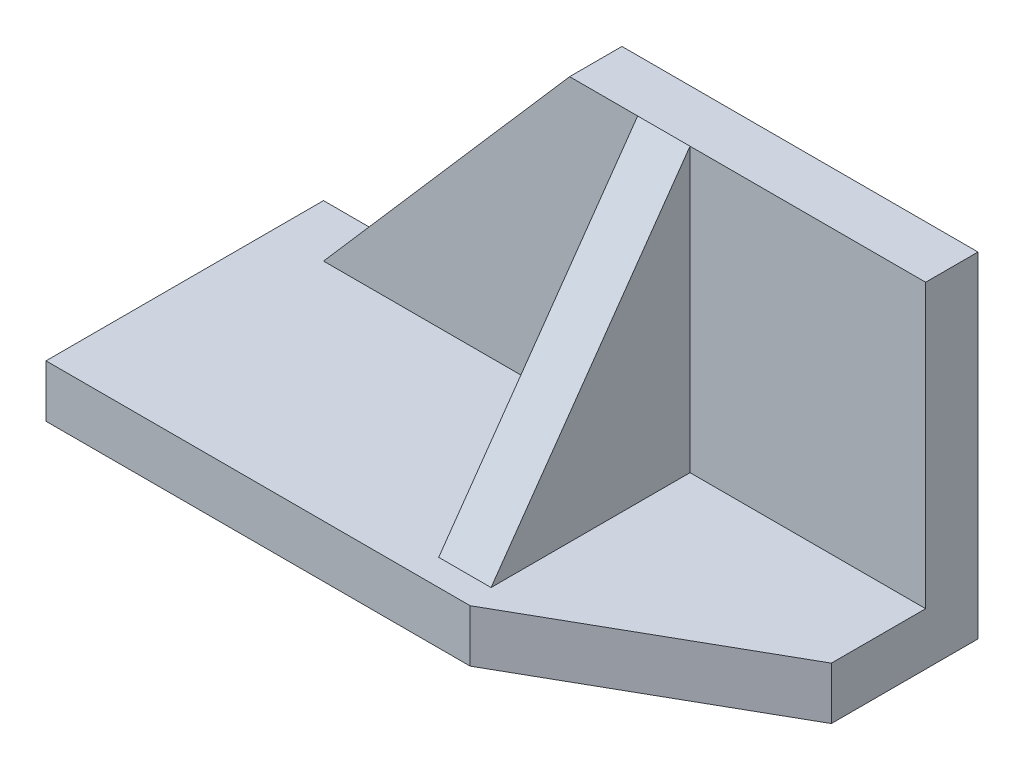
ISO-10303-21;
HEADER;
FILE_DESCRIPTION(('STEP AP214'),'2;1');
FILE_NAME('part.step','',(''),(''),'','','');
FILE_SCHEMA(('AUTOMOTIVE_DESIGN { 1 0 10303 214 1 1 1 1 }'));
ENDSEC;
DATA;
#1=APPLICATION_CONTEXT('core data for automotive mechanical design processes');
#2=APPLICATION_PROTOCOL_DEFINITION('international standard','automotive_design',2000,#1);
#3=PRODUCT_CONTEXT('',#1,'mechanical');
#4=PRODUCT('Part','Part','',(#3));
#5=PRODUCT_RELATED_PRODUCT_CATEGORY('part','',(#4));
#6=PRODUCT_DEFINITION_FORMATION('','',#4);
#7=PRODUCT_DEFINITION_CONTEXT('part definition',#1,'design');
#8=PRODUCT_DEFINITION('design','',#6,#7);
#9=PRODUCT_DEFINITION_SHAPE('','',#8);
#10=(LENGTH_UNIT() NAMED_UNIT(*) SI_UNIT(.MILLI.,.METRE.));
#11=(NAMED_UNIT(*) PLANE_ANGLE_UNIT() SI_UNIT($,.RADIAN.));
#12=(NAMED_UNIT(*) SI_UNIT($,.STERADIAN.) SOLID_ANGLE_UNIT());
#13=UNCERTAINTY_MEASURE_WITH_UNIT(LENGTH_MEASURE(1.E-05),#10,'distance_accuracy_value','');
#14=(GEOMETRIC_REPRESENTATION_CONTEXT(3) GLOBAL_UNCERTAINTY_ASSIGNED_CONTEXT((#13)) GLOBAL_UNIT_ASSIGNED_CONTEXT((#10,
#11,#12)) REPRESENTATION_CONTEXT('',''));
#15=CARTESIAN_POINT('',(0.,0.,0.));
#16=DIRECTION('',(0.,0.,1.));
#17=DIRECTION('',(1.,0.,0.));
#18=AXIS2_PLACEMENT_3D('',#15,#16,#17);
#19=CARTESIAN_POINT('',(0.,5.,0.));
#20=DIRECTION('',(0.,1.,0.));
#21=DIRECTION('',(0.,0.,1.));
#22=AXIS2_PLACEMENT_3D('',#19,#20,#21);
#23=PLANE('',#22);
#24=DIRECTION('',(1.,0.,0.));
#25=VECTOR('',#24,1.);
#26=CARTESIAN_POINT('',(80.,5.,-5.));
#27=LINE('',#26,#25);
#28=CARTESIAN_POINT('',(70.,5.,-5.));
#29=VERTEX_POINT('',#28);
#30=CARTESIAN_POINT('',(80.,5.,-5.));
#31=VERTEX_POINT('',#30);
#32=EDGE_CURVE('E53',#29,#31,#27,.T.);
#33=ORIENTED_EDGE('',*,*,#32,.F.);
#34=DIRECTION('',(0.,0.,1.));
#35=VECTOR('',#34,1.);
#36=CARTESIAN_POINT('',(70.,5.,-5.));
#37=LINE('',#36,#35);
#38=CARTESIAN_POINT('',(70.,5.,-43.));
#39=VERTEX_POINT('',#38);
#40=EDGE_CURVE('E61',#39,#29,#37,.T.);
#41=ORIENTED_EDGE('',*,*,#40,.F.);
#42=DIRECTION('',(-1.,0.,0.));
#43=VECTOR('',#42,1.);
#44=CARTESIAN_POINT('',(125.,5.,-43.));
#45=LINE('',#44,#43);
#46=CARTESIAN_POINT('',(10.,5.,-43.));
#47=VERTEX_POINT('',#46);
#48=EDGE_CURVE('E153',#39,#47,#45,.T.);
#49=ORIENTED_EDGE('',*,*,#48,.T.);
#50=DIRECTION('',(0.,0.,-1.));
#51=VECTOR('',#50,1.);
#52=CARTESIAN_POINT('',(10.,5.,-43.));
#53=LINE('',#52,#51);
#54=CARTESIAN_POINT('',(10.,5.,-53.));
#55=VERTEX_POINT('',#54);
#56=EDGE_CURVE('E164',#47,#55,#53,.T.);
#57=ORIENTED_EDGE('',*,*,#56,.T.);
#58=DIRECTION('',(-1.,0.,0.));
#59=VECTOR('',#58,1.);
#60=CARTESIAN_POINT('',(125.,5.,-53.));
#61=LINE('',#60,#59);
#62=CARTESIAN_POINT('',(0.,5.,-53.));
#63=VERTEX_POINT('',#62);
#64=EDGE_CURVE('E181',#55,#63,#61,.T.);
#65=ORIENTED_EDGE('',*,*,#64,.T.);
#66=DIRECTION('',(0.,0.,1.));
#67=VECTOR('',#66,1.);
#68=CARTESIAN_POINT('',(0.,5.,-53.));
#69=LINE('',#68,#67);
#70=CARTESIAN_POINT('',(0.,5.,0.));
#71=VERTEX_POINT('',#70);
#72=EDGE_CURVE('E172',#63,#71,#69,.T.);
#73=ORIENTED_EDGE('',*,*,#72,.T.);
#74=DIRECTION('',(1.,0.,0.));
#75=VECTOR('',#74,1.);
#76=CARTESIAN_POINT('',(0.,5.,0.));
#77=LINE('',#76,#75);
#78=CARTESIAN_POINT('',(81.,5.,0.));
#79=VERTEX_POINT('',#78);
#80=EDGE_CURVE('E175',#71,#79,#77,.T.);
#81=ORIENTED_EDGE('',*,*,#80,.T.);
#82=DIRECTION('',(0.869456557392768,0.,-0.494009407609527));
#83=VECTOR('',#82,1.);
#84=CARTESIAN_POINT('',(81.,5.,0.));
#85=LINE('',#84,#83);
#86=CARTESIAN_POINT('',(125.,5.,-25.));
#87=VERTEX_POINT('',#86);
#88=EDGE_CURVE('E177',#79,#87,#85,.T.);
#89=ORIENTED_EDGE('',*,*,#88,.T.);
#90=DIRECTION('',(0.,0.,-1.));
#91=VECTOR('',#90,1.);
#92=CARTESIAN_POINT('',(125.,5.,-25.));
#93=LINE('',#92,#91);
#94=CARTESIAN_POINT('',(125.,5.,-43.));
#95=VERTEX_POINT('',#94);
#96=EDGE_CURVE('E176',#87,#95,#93,.T.);
#97=ORIENTED_EDGE('',*,*,#96,.T.);
#98=CARTESIAN_POINT('',(80.,5.,-43.));
#99=VERTEX_POINT('',#98);
#100=EDGE_CURVE('E152',#95,#99,#45,.T.);
#101=ORIENTED_EDGE('',*,*,#100,.T.);
#102=DIRECTION('',(0.,0.,-1.));
#103=VECTOR('',#102,1.);
#104=CARTESIAN_POINT('',(80.,5.,-43.));
#105=LINE('',#104,#103);
#106=EDGE_CURVE('E132',#31,#99,#105,.T.);
#107=ORIENTED_EDGE('',*,*,#106,.F.);
#108=EDGE_LOOP('',(#33,#41,#49,#57,#65,#73,#81,#89,#97,#101,#107));
#109=FACE_BOUND('',#108,.T.);
#110=ADVANCED_FACE('F39',(#109),#23,.T.);
#111=CARTESIAN_POINT('',(0.,0.,-43.));
#112=DIRECTION('',(0.,0.,-1.));
#113=DIRECTION('',(-1.,0.,0.));
#114=AXIS2_PLACEMENT_3D('',#111,#112,#113);
#115=PLANE('',#114);
#116=DIRECTION('',(0.,-1.,0.));
#117=VECTOR('',#116,1.);
#118=CARTESIAN_POINT('',(70.,59.,-43.));
#119=LINE('',#118,#117);
#120=CARTESIAN_POINT('',(70.,59.,-43.));
#121=VERTEX_POINT('',#120);
#122=EDGE_CURVE('E138',#121,#39,#119,.T.);
#123=ORIENTED_EDGE('',*,*,#122,.F.);
#124=DIRECTION('',(-1.,0.,0.));
#125=VECTOR('',#124,1.);
#126=CARTESIAN_POINT('',(125.,59.,-43.));
#127=LINE('',#126,#125);
#128=CARTESIAN_POINT('',(57.,59.,-43.));
#129=VERTEX_POINT('',#128);
#130=EDGE_CURVE('E147',#121,#129,#127,.T.);
#131=ORIENTED_EDGE('',*,*,#130,.T.);
#132=DIRECTION('',(-0.656524478023403,-0.754304719431145,0.));
#133=VECTOR('',#132,1.);
#134=CARTESIAN_POINT('',(57.,59.,-43.));
#135=LINE('',#134,#133);
#136=EDGE_CURVE('E149',#129,#47,#135,.T.);
#137=ORIENTED_EDGE('',*,*,#136,.T.);
#138=ORIENTED_EDGE('',*,*,#48,.F.);
#139=EDGE_LOOP('',(#123,#131,#137,#138));
#140=FACE_BOUND('',#139,.T.);
#141=ADVANCED_FACE('F241',(#140),#115,.F.);
#142=DIRECTION('',(0.,-1.,0.));
#143=VECTOR('',#142,1.);
#144=CARTESIAN_POINT('',(80.,59.,-43.));
#145=LINE('',#144,#143);
#146=CARTESIAN_POINT('',(80.,59.,-43.));
#147=VERTEX_POINT('',#146);
#148=EDGE_CURVE('E142',#147,#99,#145,.T.);
#149=ORIENTED_EDGE('',*,*,#148,.T.);
#150=ORIENTED_EDGE('',*,*,#100,.F.);
#151=DIRECTION('',(0.,1.,0.));
#152=VECTOR('',#151,1.);
#153=CARTESIAN_POINT('',(125.,5.,-43.));
#154=LINE('',#153,#152);
#155=CARTESIAN_POINT('',(125.,59.,-43.));
#156=VERTEX_POINT('',#155);
#157=EDGE_CURVE('E156',#95,#156,#154,.T.);
#158=ORIENTED_EDGE('',*,*,#157,.T.);
#159=EDGE_CURVE('E148',#156,#147,#127,.T.);
#160=ORIENTED_EDGE('',*,*,#159,.T.);
#161=EDGE_LOOP('',(#149,#150,#158,#160));
#162=FACE_BOUND('',#161,.T.);
#163=ADVANCED_FACE('F230',(#162),#115,.F.);
#164=CARTESIAN_POINT('',(0.,5.,-53.));
#165=DIRECTION('',(1.,0.,0.));
#166=DIRECTION('',(0.,0.,-1.));
#167=AXIS2_PLACEMENT_3D('',#164,#165,#166);
#168=PLANE('',#167);
#169=DIRECTION('',(0.,0.,1.));
#170=VECTOR('',#169,1.);
#171=CARTESIAN_POINT('',(0.,-5.,-53.));
#172=LINE('',#171,#170);
#173=CARTESIAN_POINT('',(0.,-5.,-53.));
#174=VERTEX_POINT('',#173);
#175=CARTESIAN_POINT('',(0.,-5.,0.));
#176=VERTEX_POINT('',#175);
#177=EDGE_CURVE('E171',#174,#176,#172,.T.);
#178=ORIENTED_EDGE('',*,*,#177,.T.);
#179=DIRECTION('',(0.,-1.,0.));
#180=VECTOR('',#179,1.);
#181=CARTESIAN_POINT('',(0.,5.,0.));
#182=LINE('',#181,#180);
#183=EDGE_CURVE('E11',#71,#176,#182,.T.);
#184=ORIENTED_EDGE('',*,*,#183,.F.);
#185=ORIENTED_EDGE('',*,*,#72,.F.);
#186=DIRECTION('',(0.,-1.,0.));
#187=VECTOR('',#186,1.);
#188=CARTESIAN_POINT('',(0.,5.,-53.));
#189=LINE('',#188,#187);
#190=EDGE_CURVE('E183',#63,#174,#189,.T.);
#191=ORIENTED_EDGE('',*,*,#190,.T.);
#192=EDGE_LOOP('',(#178,#184,#185,#191));
#193=FACE_BOUND('',#192,.T.);
#194=ADVANCED_FACE('F41',(#193),#168,.F.);
#195=CARTESIAN_POINT('',(0.,5.,0.));
#196=DIRECTION('',(0.,0.,-1.));
#197=DIRECTION('',(-1.,0.,0.));
#198=AXIS2_PLACEMENT_3D('',#195,#196,#197);
#199=PLANE('',#198);
#200=DIRECTION('',(1.,0.,0.));
#201=VECTOR('',#200,1.);
#202=CARTESIAN_POINT('',(0.,-5.,0.));
#203=LINE('',#202,#201);
#204=CARTESIAN_POINT('',(81.,-5.,0.));
#205=VERTEX_POINT('',#204);
#206=EDGE_CURVE('E189',#176,#205,#203,.T.);
#207=ORIENTED_EDGE('',*,*,#206,.T.);
#208=DIRECTION('',(0.,-1.,0.));
#209=VECTOR('',#208,1.);
#210=CARTESIAN_POINT('',(81.,5.,0.));
#211=LINE('',#210,#209);
#212=EDGE_CURVE('E50',#79,#205,#211,.T.);
#213=ORIENTED_EDGE('',*,*,#212,.F.);
#214=ORIENTED_EDGE('',*,*,#80,.F.);
#215=ORIENTED_EDGE('',*,*,#183,.T.);
#216=EDGE_LOOP('',(#207,#213,#214,#215));
#217=FACE_BOUND('',#216,.T.);
#218=ADVANCED_FACE('F235',(#217),#199,.F.);
#219=CARTESIAN_POINT('',(81.,5.,0.));
#220=DIRECTION('',(-0.494009407609527,0.,-0.869456557392768));
#221=DIRECTION('',(-0.869456557392768,0.,0.494009407609528));
#222=AXIS2_PLACEMENT_3D('',#219,#220,#221);
#223=PLANE('',#222);
#224=DIRECTION('',(0.869456557392768,0.,-0.494009407609527));
#225=VECTOR('',#224,1.);
#226=CARTESIAN_POINT('',(81.,-5.,0.));
#227=LINE('',#226,#225);
#228=CARTESIAN_POINT('',(125.,-5.,-25.));
#229=VERTEX_POINT('',#228);
#230=EDGE_CURVE('E190',#205,#229,#227,.T.);
#231=ORIENTED_EDGE('',*,*,#230,.T.);
#232=DIRECTION('',(0.,-1.,0.));
#233=VECTOR('',#232,1.);
#234=CARTESIAN_POINT('',(125.,5.,-25.));
#235=LINE('',#234,#233);
#236=EDGE_CURVE('E199',#87,#229,#235,.T.);
#237=ORIENTED_EDGE('',*,*,#236,.F.);
#238=ORIENTED_EDGE('',*,*,#88,.F.);
#239=ORIENTED_EDGE('',*,*,#212,.T.);
#240=EDGE_LOOP('',(#231,#237,#238,#239));
#241=FACE_BOUND('',#240,.T.);
#242=ADVANCED_FACE('F210',(#241),#223,.F.);
#243=CARTESIAN_POINT('',(125.,5.,-25.));
#244=DIRECTION('',(-1.,0.,0.));
#245=DIRECTION('',(0.,0.,1.));
#246=AXIS2_PLACEMENT_3D('',#243,#244,#245);
#247=PLANE('',#246);
#248=DIRECTION('',(0.,0.,-1.));
#249=VECTOR('',#248,1.);
#250=CARTESIAN_POINT('',(125.,-5.,-25.));
#251=LINE('',#250,#249);
#252=CARTESIAN_POINT('',(125.,-5.,-53.));
#253=VERTEX_POINT('',#252);
#254=EDGE_CURVE('E194',#229,#253,#251,.T.);
#255=ORIENTED_EDGE('',*,*,#254,.T.);
#256=DIRECTION('',(0.,-1.,0.));
#257=VECTOR('',#256,1.);
#258=CARTESIAN_POINT('',(125.,5.,-53.));
#259=LINE('',#258,#257);
#260=CARTESIAN_POINT('',(125.,59.,-53.));
#261=VERTEX_POINT('',#260);
#262=EDGE_CURVE('E197',#261,#253,#259,.T.);
#263=ORIENTED_EDGE('',*,*,#262,.F.);
#264=DIRECTION('',(0.,0.,-1.));
#265=VECTOR('',#264,1.);
#266=CARTESIAN_POINT('',(125.,59.,-43.));
#267=LINE('',#266,#265);
#268=EDGE_CURVE('E158',#156,#261,#267,.T.);
#269=ORIENTED_EDGE('',*,*,#268,.F.);
#270=ORIENTED_EDGE('',*,*,#157,.F.);
#271=ORIENTED_EDGE('',*,*,#96,.F.);
#272=ORIENTED_EDGE('',*,*,#236,.T.);
#273=EDGE_LOOP('',(#255,#263,#269,#270,#271,#272));
#274=FACE_BOUND('',#273,.T.);
#275=ADVANCED_FACE('F216',(#274),#247,.F.);
#276=CARTESIAN_POINT('',(125.,5.,-53.));
#277=DIRECTION('',(0.,0.,1.));
#278=DIRECTION('',(1.,0.,0.));
#279=AXIS2_PLACEMENT_3D('',#276,#277,#278);
#280=PLANE('',#279);
#281=DIRECTION('',(-1.,0.,0.));
#282=VECTOR('',#281,1.);
#283=CARTESIAN_POINT('',(125.,-5.,-53.));
#284=LINE('',#283,#282);
#285=EDGE_CURVE('E178',#253,#174,#284,.T.);
#286=ORIENTED_EDGE('',*,*,#285,.T.);
#287=ORIENTED_EDGE('',*,*,#190,.F.);
#288=ORIENTED_EDGE('',*,*,#64,.F.);
#289=DIRECTION('',(-0.656524478023403,-0.754304719431145,0.));
#290=VECTOR('',#289,1.);
#291=CARTESIAN_POINT('',(57.,59.,-53.));
#292=LINE('',#291,#290);
#293=CARTESIAN_POINT('',(57.,59.,-53.));
#294=VERTEX_POINT('',#293);
#295=EDGE_CURVE('E161',#294,#55,#292,.T.);
#296=ORIENTED_EDGE('',*,*,#295,.F.);
#297=DIRECTION('',(-1.,0.,0.));
#298=VECTOR('',#297,1.);
#299=CARTESIAN_POINT('',(125.,59.,-53.));
#300=LINE('',#299,#298);
#301=EDGE_CURVE('E144',#261,#294,#300,.T.);
#302=ORIENTED_EDGE('',*,*,#301,.F.);
#303=ORIENTED_EDGE('',*,*,#262,.T.);
#304=EDGE_LOOP('',(#286,#287,#288,#296,#302,#303));
#305=FACE_BOUND('',#304,.T.);
#306=ADVANCED_FACE('F222',(#305),#280,.F.);
#307=CARTESIAN_POINT('',(0.,-5.,0.));
#308=DIRECTION('',(0.,1.,0.));
#309=DIRECTION('',(0.,0.,1.));
#310=AXIS2_PLACEMENT_3D('',#307,#308,#309);
#311=PLANE('',#310);
#312=ORIENTED_EDGE('',*,*,#177,.F.);
#313=ORIENTED_EDGE('',*,*,#285,.F.);
#314=ORIENTED_EDGE('',*,*,#254,.F.);
#315=ORIENTED_EDGE('',*,*,#230,.F.);
#316=ORIENTED_EDGE('',*,*,#206,.F.);
#317=EDGE_LOOP('',(#312,#313,#314,#315,#316));
#318=FACE_BOUND('',#317,.T.);
#319=ADVANCED_FACE('F213',(#318),#311,.F.);
#320=CARTESIAN_POINT('',(125.,59.,-43.));
#321=DIRECTION('',(0.,-1.,0.));
#322=DIRECTION('',(0.,0.,-1.));
#323=AXIS2_PLACEMENT_3D('',#320,#321,#322);
#324=PLANE('',#323);
#325=ORIENTED_EDGE('',*,*,#130,.F.);
#326=DIRECTION('',(1.,0.,0.));
#327=VECTOR('',#326,1.);
#328=CARTESIAN_POINT('',(70.,59.,-43.));
#329=LINE('',#328,#327);
#330=EDGE_CURVE('E122',#121,#147,#329,.T.);
#331=ORIENTED_EDGE('',*,*,#330,.T.);
#332=ORIENTED_EDGE('',*,*,#159,.F.);
#333=ORIENTED_EDGE('',*,*,#268,.T.);
#334=ORIENTED_EDGE('',*,*,#301,.T.);
#335=DIRECTION('',(0.,0.,-1.));
#336=VECTOR('',#335,1.);
#337=CARTESIAN_POINT('',(57.,59.,-43.));
#338=LINE('',#337,#336);
#339=EDGE_CURVE('E169',#129,#294,#338,.T.);
#340=ORIENTED_EDGE('',*,*,#339,.F.);
#341=EDGE_LOOP('',(#325,#331,#332,#333,#334,#340));
#342=FACE_BOUND('',#341,.T.);
#343=ADVANCED_FACE('F226',(#342),#324,.F.);
#344=CARTESIAN_POINT('',(57.,59.,-43.));
#345=DIRECTION('',(0.754304719431145,-0.656524478023403,0.));
#346=DIRECTION('',(0.656524478023403,0.754304719431145,0.));
#347=AXIS2_PLACEMENT_3D('',#344,#345,#346);
#348=PLANE('',#347);
#349=ORIENTED_EDGE('',*,*,#295,.T.);
#350=ORIENTED_EDGE('',*,*,#56,.F.);
#351=ORIENTED_EDGE('',*,*,#136,.F.);
#352=ORIENTED_EDGE('',*,*,#339,.T.);
#353=EDGE_LOOP('',(#349,#350,#351,#352));
#354=FACE_BOUND('',#353,.T.);
#355=ADVANCED_FACE('F239',(#354),#348,.F.);
#356=CARTESIAN_POINT('',(70.,59.,-5.));
#357=DIRECTION('',(1.,0.,0.));
#358=DIRECTION('',(0.,0.,-1.));
#359=AXIS2_PLACEMENT_3D('',#356,#357,#358);
#360=PLANE('',#359);
#361=ORIENTED_EDGE('',*,*,#40,.T.);
#362=DIRECTION('',(0.,0.817806419300767,-0.575493406174614));
#363=VECTOR('',#362,1.);
#364=CARTESIAN_POINT('',(70.,59.,-43.));
#365=LINE('',#364,#363);
#366=EDGE_CURVE('E120',#29,#121,#365,.T.);
#367=ORIENTED_EDGE('',*,*,#366,.T.);
#368=ORIENTED_EDGE('',*,*,#122,.T.);
#369=EDGE_LOOP('',(#361,#367,#368));
#370=FACE_BOUND('',#369,.T.);
#371=ADVANCED_FACE('F133',(#370),#360,.F.);
#372=CARTESIAN_POINT('',(80.,59.,-43.));
#373=DIRECTION('',(-1.,0.,0.));
#374=DIRECTION('',(0.,0.,1.));
#375=AXIS2_PLACEMENT_3D('',#372,#373,#374);
#376=PLANE('',#375);
#377=ORIENTED_EDGE('',*,*,#148,.F.);
#378=DIRECTION('',(0.,0.817806419300767,-0.575493406174614));
#379=VECTOR('',#378,1.);
#380=CARTESIAN_POINT('',(80.,59.,-43.));
#381=LINE('',#380,#379);
#382=EDGE_CURVE('E130',#31,#147,#381,.T.);
#383=ORIENTED_EDGE('',*,*,#382,.F.);
#384=ORIENTED_EDGE('',*,*,#106,.T.);
#385=EDGE_LOOP('',(#377,#383,#384));
#386=FACE_BOUND('',#385,.T.);
#387=ADVANCED_FACE('F244',(#386),#376,.F.);
#388=CARTESIAN_POINT('',(70.,59.,-43.));
#389=DIRECTION('',(0.,-0.575493406174614,-0.817806419300767));
#390=DIRECTION('',(0.,0.817806419300767,-0.575493406174613));
#391=AXIS2_PLACEMENT_3D('',#388,#389,#390);
#392=PLANE('',#391);
#393=ORIENTED_EDGE('',*,*,#382,.T.);
#394=ORIENTED_EDGE('',*,*,#330,.F.);
#395=ORIENTED_EDGE('',*,*,#366,.F.);
#396=ORIENTED_EDGE('',*,*,#32,.T.);
#397=EDGE_LOOP('',(#393,#394,#395,#396));
#398=FACE_BOUND('',#397,.T.);
#399=ADVANCED_FACE('F123',(#398),#392,.F.);
#400=CLOSED_SHELL('',(#110,#141,#163,#194,#218,#242,#275,#306,#319,#343,#355,#371,#387,#399));
#401=MANIFOLD_SOLID_BREP('B2',#400);
#402=ADVANCED_BREP_SHAPE_REPRESENTATION('',(#18,#401),#14);
#403=SHAPE_DEFINITION_REPRESENTATION(#9,#402);
ENDSEC;
END-ISO-10303-21;
